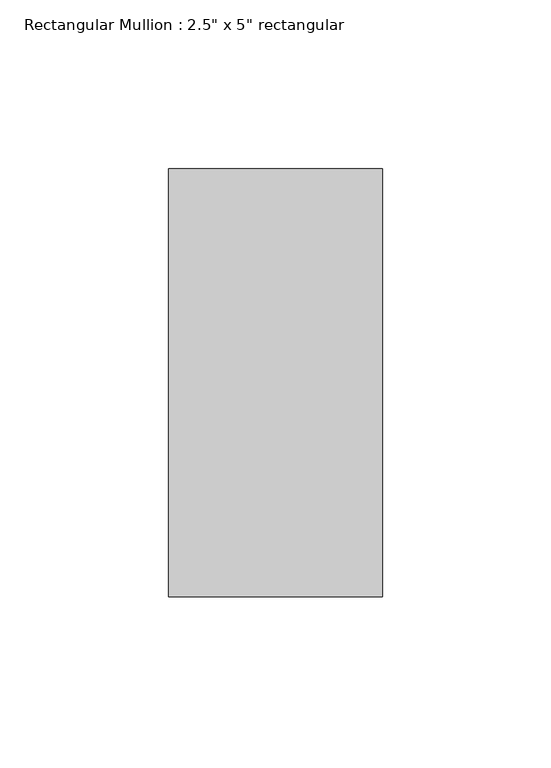
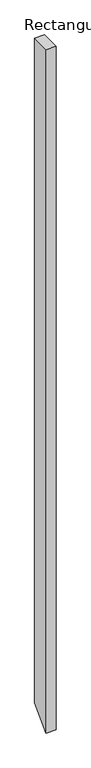
"""IFC4 building model written with IfcOpenShell, lengths in millimetres: member geometry."""

from ifc_helpers import new_model, si_unit, frame, origin, place, context, project, spatial, polyline, outline, extrude, source, transform, mapped, element, save


def member_a84de01e(model_context):
    return source(origin(), model_context, "Body", "SweptSolid", [
        extrude(outline(polyline([(-63.5, 0.0), (63.5, 0.0), (63.5, -4484.3796866), (-63.5, -4611.3796866), (-63.5, 0.0)])), frame((-63.5, 0.0, 0.0), z_axis=(1.0, 0.0, 0.0), x_axis=(0.0, 1.0, 0.0)), (0.0, 0.0, 1.0), 63.5),
    ])


if __name__ == "__main__":
    model = new_model("IFC4")
    model_context = context("Model", 3, world=origin())
    ifc_project = project(units=[si_unit("LENGTHUNIT", "METRE", prefix="MILLI")], contexts=[model_context])
    site = spatial("IfcSite", under=ifc_project)
    building = spatial("IfcBuilding", under=site)
    placement = place(None, origin())
    member_shape = member_a84de01e(model_context)
    element("IfcMember", 1, ObjectType="Rectangular Mullion : 2.5\" x 5\" rectangular", at=placement, inside=building, context=model_context, shape_type="MappedRepresentation", body=[
        mapped(member_shape, transform((0.0, 0.0, 0.0), x_axis=(1.0, 0.0, 0.0), y_axis=(0.0, 1.0, 0.0), z_axis=(0.0, 0.0, 1.0))),
    ])
    save(model, "model.ifc")

# Revit data of these elements
# Type "Rectangular Mullion : 2.5\" x 5\" rectangular"
#   built-in parameter 1007304 = 0.416667 (stored number, unit not read)
#   built-in parameter 1007301 = 0.104167 (stored number, unit not read)
#   built-in parameter 1007300 = 0.104167 (stored number, unit not read)
# Element 1 (IfcMember, "Rectangular Mullion : 2.5\" x 5\" rectangular")
#   Materials on its faces: "Aluminum"
# Materials
#   "Aluminum": class "Metal", colour RGB 247 247 247, transparency 0, Description = "Aluminum 6061", Cost = 0
